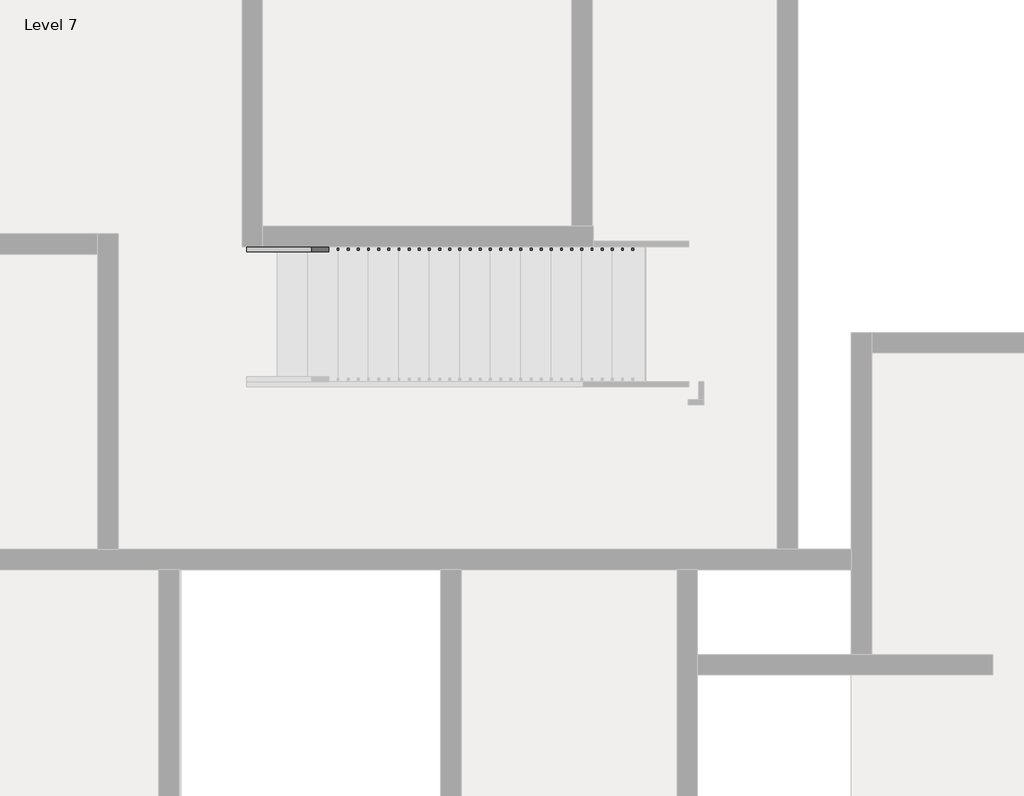
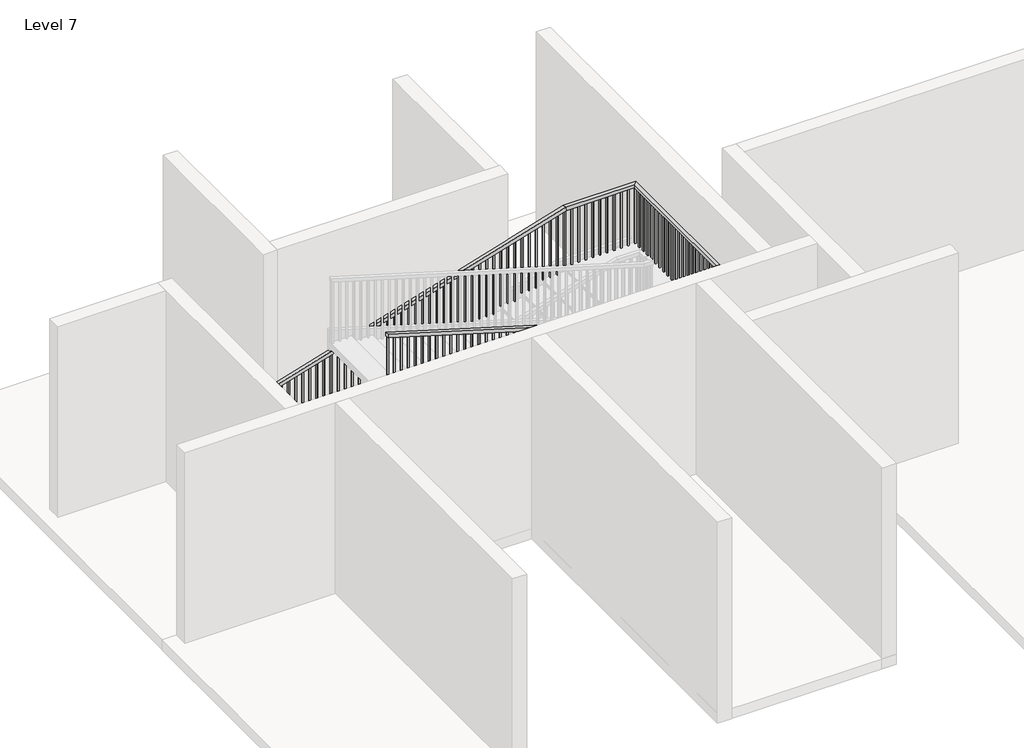
# One storey, part 10 of 14: 1 railing.
"""IFC4 building model written with IfcOpenShell, lengths in millimetres."""

from ifc_helpers import new_model, si_unit, frame, origin, place, context, project, spatial, polyline, outline, extrude, faceted_brep, element, save

model = new_model("IFC4")

# Units and contexts
model_context = context("Model", 3, world=origin())
ifc_project = project(units=[si_unit("LENGTHUNIT", "METRE", prefix="MILLI")], contexts=[model_context])

# Site, building, storey
site = spatial("IfcSite", under=ifc_project)
building = spatial("IfcBuilding", under=site)
storey = spatial("IfcBuildingStorey", under=building, Name="Level 7", Elevation=18288.0)

# Railing
placement = place(None, origin())
element("IfcRailing", 1, ObjectType="Handrail - Rectangular", at=placement, inside=storey, context=model_context, shape_type="SolidModel", body=[
    faceted_brep([(-5254.0891351, 12506.0715905, 19293.84), (-5254.0891351, 12506.0715905, 19240.8032429), (-5254.0891351, 12455.2715905, 19240.8032429), (-5254.0891351, 12455.2715905, 19293.84), (-986.8891351, 12506.0715905, 20574.0), (-979.4332782, 12506.0715905, 20523.2), (-979.4332782, 12455.2715905, 20523.2), (-986.8891351, 12455.2715905, 20574.0), (54.5108649, 12506.0715905, 20574.0), (54.5108649, 12506.0715905, 20523.2), (3.7108649, 12455.2715905, 20523.2), (3.7108649, 12455.2715905, 20574.0), (54.5108649, 9478.4949943, 20574.0), (54.5108649, 9478.4949943, 20523.2), (3.7108649, 9529.2949943, 20523.2), (3.7108649, 9529.2949943, 20574.0), (-682.0891351, 9478.4949943, 20574.0), (-689.544992, 9478.4949943, 20523.2), (-689.544992, 9529.2949943, 20523.2), (-682.0891351, 9529.2949943, 20574.0), (-5254.0891351, 9478.4949943, 21945.6), (-5254.0891351, 9529.2949943, 21945.6), (-5254.0891351, 9529.2949943, 21892.5632429), (-5254.0891351, 9478.4949943, 21892.5632429)], [[[0, 1, 2, 3]], [[1, 0, 4, 5]], [[2, 1, 5, 6]], [[3, 2, 6, 7]], [[0, 3, 7, 4]], [[5, 4, 8, 9]], [[6, 5, 9, 10]], [[7, 6, 10, 11]], [[4, 7, 11, 8]], [[9, 8, 12, 13]], [[10, 9, 13, 14]], [[11, 10, 14, 15]], [[8, 11, 15, 12]], [[13, 12, 16, 17]], [[14, 13, 17, 18]], [[15, 14, 18, 19]], [[12, 15, 19, 16]], [[20, 21, 22, 23]], [[17, 16, 20, 23]], [[18, 17, 23, 22]], [[19, 18, 22, 21]], [[16, 19, 21, 20]]]),
    extrude(outline(polyline([(21864.9407429, -5162.0141351), (20939.76, -5162.0141351), (20939.76, -5142.9641351), (21859.2257429, -5142.9641351), (21864.9407429, -5162.0141351)])), frame((0.0, 9494.3699943, 0.0), z_axis=(0.0, 1.0, 0.0), x_axis=(0.0, 0.0, 1.0)), (0.0, 0.0, 1.0), 19.05),
    extrude(outline(polyline([(21834.4607429, -5060.4141351), (20939.76, -5060.4141351), (20939.76, -5041.3641351), (21828.7457429, -5041.3641351), (21834.4607429, -5060.4141351)])), frame((0.0, 9494.3699943, 0.0), z_axis=(0.0, 1.0, 0.0), x_axis=(0.0, 0.0, 1.0)), (0.0, 0.0, 1.0), 19.05),
    extrude(outline(polyline([(21803.9807429, -4958.8141351), (20939.76, -4958.8141351), (20939.76, -4939.7641351), (21798.2657429, -4939.7641351), (21803.9807429, -4958.8141351)])), frame((0.0, 9494.3699943, 0.0), z_axis=(0.0, 1.0, 0.0), x_axis=(0.0, 0.0, 1.0)), (0.0, 0.0, 1.0), 19.05),
    extrude(outline(polyline([(21773.5007429, -4857.2141351), (20848.32, -4857.2141351), (20848.32, -4838.1641351), (21767.7857429, -4838.1641351), (21773.5007429, -4857.2141351)])), frame((0.0, 9494.3699943, 0.0), z_axis=(0.0, 1.0, 0.0), x_axis=(0.0, 0.0, 1.0)), (0.0, 0.0, 1.0), 19.05),
    extrude(outline(polyline([(21743.0207429, -4755.6141351), (20848.32, -4755.6141351), (20848.32, -4736.5641351), (21737.3057429, -4736.5641351), (21743.0207429, -4755.6141351)])), frame((0.0, 9494.3699943, 0.0), z_axis=(0.0, 1.0, 0.0), x_axis=(0.0, 0.0, 1.0)), (0.0, 0.0, 1.0), 19.05),
    extrude(outline(polyline([(21712.5407429, -4654.0141351), (20848.32, -4654.0141351), (20848.32, -4634.9641351), (21706.8257429, -4634.9641351), (21712.5407429, -4654.0141351)])), frame((0.0, 9494.3699943, 0.0), z_axis=(0.0, 1.0, 0.0), x_axis=(0.0, 0.0, 1.0)), (0.0, 0.0, 1.0), 19.05),
    extrude(outline(polyline([(21682.0607429, -4552.4141351), (20756.88, -4552.4141351), (20756.88, -4533.3641351), (21676.3457429, -4533.3641351), (21682.0607429, -4552.4141351)])), frame((0.0, 9494.3699943, 0.0), z_axis=(0.0, 1.0, 0.0), x_axis=(0.0, 0.0, 1.0)), (0.0, 0.0, 1.0), 19.05),
    extrude(outline(polyline([(21651.5807429, -4450.8141351), (20756.88, -4450.8141351), (20756.88, -4431.7641351), (21645.8657429, -4431.7641351), (21651.5807429, -4450.8141351)])), frame((0.0, 9494.3699943, 0.0), z_axis=(0.0, 1.0, 0.0), x_axis=(0.0, 0.0, 1.0)), (0.0, 0.0, 1.0), 19.05),
    extrude(outline(polyline([(21621.1007429, -4349.2141351), (20756.88, -4349.2141351), (20756.88, -4330.1641351), (21615.3857429, -4330.1641351), (21621.1007429, -4349.2141351)])), frame((0.0, 9494.3699943, 0.0), z_axis=(0.0, 1.0, 0.0), x_axis=(0.0, 0.0, 1.0)), (0.0, 0.0, 1.0), 19.05),
    extrude(outline(polyline([(21590.6207429, -4247.6141351), (20665.44, -4247.6141351), (20665.44, -4228.5641351), (21584.9057429, -4228.5641351), (21590.6207429, -4247.6141351)])), frame((0.0, 9494.3699943, 0.0), z_axis=(0.0, 1.0, 0.0), x_axis=(0.0, 0.0, 1.0)), (0.0, 0.0, 1.0), 19.05),
    extrude(outline(polyline([(21560.1407429, -4146.0141351), (20665.44, -4146.0141351), (20665.44, -4126.9641351), (21554.4257429, -4126.9641351), (21560.1407429, -4146.0141351)])), frame((0.0, 9494.3699943, 0.0), z_axis=(0.0, 1.0, 0.0), x_axis=(0.0, 0.0, 1.0)), (0.0, 0.0, 1.0), 19.05),
    extrude(outline(polyline([(21529.6607429, -4044.4141351), (20665.44, -4044.4141351), (20665.44, -4025.3641351), (21523.9457429, -4025.3641351), (21529.6607429, -4044.4141351)])), frame((0.0, 9494.3699943, 0.0), z_axis=(0.0, 1.0, 0.0), x_axis=(0.0, 0.0, 1.0)), (0.0, 0.0, 1.0), 19.05),
    extrude(outline(polyline([(21499.1807429, -3942.8141351), (20574.0, -3942.8141351), (20574.0, -3923.7641351), (21493.4657429, -3923.7641351), (21499.1807429, -3942.8141351)])), frame((0.0, 9494.3699943, 0.0), z_axis=(0.0, 1.0, 0.0), x_axis=(0.0, 0.0, 1.0)), (0.0, 0.0, 1.0), 19.05),
    extrude(outline(polyline([(21468.7007429, -3841.2141351), (20574.0, -3841.2141351), (20574.0, -3822.1641351), (21462.9857429, -3822.1641351), (21468.7007429, -3841.2141351)])), frame((0.0, 9494.3699943, 0.0), z_axis=(0.0, 1.0, 0.0), x_axis=(0.0, 0.0, 1.0)), (0.0, 0.0, 1.0), 19.05),
    extrude(outline(polyline([(21438.2207429, -3739.6141351), (20574.0, -3739.6141351), (20574.0, -3720.5641351), (21432.5057429, -3720.5641351), (21438.2207429, -3739.6141351)])), frame((0.0, 9494.3699943, 0.0), z_axis=(0.0, 1.0, 0.0), x_axis=(0.0, 0.0, 1.0)), (0.0, 0.0, 1.0), 19.05),
    extrude(outline(polyline([(21407.7407429, -3638.0141351), (20482.56, -3638.0141351), (20482.56, -3618.9641351), (21402.0257429, -3618.9641351), (21407.7407429, -3638.0141351)])), frame((0.0, 9494.3699943, 0.0), z_axis=(0.0, 1.0, 0.0), x_axis=(0.0, 0.0, 1.0)), (0.0, 0.0, 1.0), 19.05),
    extrude(outline(polyline([(21377.2607429, -3536.4141351), (20482.56, -3536.4141351), (20482.56, -3517.3641351), (21371.5457429, -3517.3641351), (21377.2607429, -3536.4141351)])), frame((0.0, 9494.3699943, 0.0), z_axis=(0.0, 1.0, 0.0), x_axis=(0.0, 0.0, 1.0)), (0.0, 0.0, 1.0), 19.05),
    extrude(outline(polyline([(21346.7807429, -3434.8141351), (20482.56, -3434.8141351), (20482.56, -3415.7641351), (21341.0657429, -3415.7641351), (21346.7807429, -3434.8141351)])), frame((0.0, 9494.3699943, 0.0), z_axis=(0.0, 1.0, 0.0), x_axis=(0.0, 0.0, 1.0)), (0.0, 0.0, 1.0), 19.05),
    extrude(outline(polyline([(21316.3007429, -3333.2141351), (20391.12, -3333.2141351), (20391.12, -3314.1641351), (21310.5857429, -3314.1641351), (21316.3007429, -3333.2141351)])), frame((0.0, 9494.3699943, 0.0), z_axis=(0.0, 1.0, 0.0), x_axis=(0.0, 0.0, 1.0)), (0.0, 0.0, 1.0), 19.05),
    extrude(outline(polyline([(21285.8207429, -3231.6141351), (20391.12, -3231.6141351), (20391.12, -3212.5641351), (21280.1057429, -3212.5641351), (21285.8207429, -3231.6141351)])), frame((0.0, 9494.3699943, 0.0), z_axis=(0.0, 1.0, 0.0), x_axis=(0.0, 0.0, 1.0)), (0.0, 0.0, 1.0), 19.05),
    extrude(outline(polyline([(21255.3407429, -3130.0141351), (20391.12, -3130.0141351), (20391.12, -3110.9641351), (21249.6257429, -3110.9641351), (21255.3407429, -3130.0141351)])), frame((0.0, 9494.3699943, 0.0), z_axis=(0.0, 1.0, 0.0), x_axis=(0.0, 0.0, 1.0)), (0.0, 0.0, 1.0), 19.05),
    extrude(outline(polyline([(21224.8607429, -3028.4141351), (20299.68, -3028.4141351), (20299.68, -3009.3641351), (21219.1457429, -3009.3641351), (21224.8607429, -3028.4141351)])), frame((0.0, 9494.3699943, 0.0), z_axis=(0.0, 1.0, 0.0), x_axis=(0.0, 0.0, 1.0)), (0.0, 0.0, 1.0), 19.05),
    extrude(outline(polyline([(21194.3807429, -2926.8141351), (20299.68, -2926.8141351), (20299.68, -2907.7641351), (21188.6657429, -2907.7641351), (21194.3807429, -2926.8141351)])), frame((0.0, 9494.3699943, 0.0), z_axis=(0.0, 1.0, 0.0), x_axis=(0.0, 0.0, 1.0)), (0.0, 0.0, 1.0), 19.05),
    extrude(outline(polyline([(21163.9007429, -2825.2141351), (20299.68, -2825.2141351), (20299.68, -2806.1641351), (21158.1857429, -2806.1641351), (21163.9007429, -2825.2141351)])), frame((0.0, 9494.3699943, 0.0), z_axis=(0.0, 1.0, 0.0), x_axis=(0.0, 0.0, 1.0)), (0.0, 0.0, 1.0), 19.05),
    extrude(outline(polyline([(21133.4207429, -2723.6141351), (20208.24, -2723.6141351), (20208.24, -2704.5641351), (21127.7057429, -2704.5641351), (21133.4207429, -2723.6141351)])), frame((0.0, 9494.3699943, 0.0), z_axis=(0.0, 1.0, 0.0), x_axis=(0.0, 0.0, 1.0)), (0.0, 0.0, 1.0), 19.05),
    extrude(outline(polyline([(21102.9407429, -2622.0141351), (20208.24, -2622.0141351), (20208.24, -2602.9641351), (21097.2257429, -2602.9641351), (21102.9407429, -2622.0141351)])), frame((0.0, 9494.3699943, 0.0), z_axis=(0.0, 1.0, 0.0), x_axis=(0.0, 0.0, 1.0)), (0.0, 0.0, 1.0), 19.05),
    extrude(outline(polyline([(21072.4607429, -2520.4141351), (20208.24, -2520.4141351), (20208.24, -2501.3641351), (21066.7457429, -2501.3641351), (21072.4607429, -2520.4141351)])), frame((0.0, 9494.3699943, 0.0), z_axis=(0.0, 1.0, 0.0), x_axis=(0.0, 0.0, 1.0)), (0.0, 0.0, 1.0), 19.05),
    extrude(outline(polyline([(21041.9807429, -2418.8141351), (20116.8, -2418.8141351), (20116.8, -2399.7641351), (21036.2657429, -2399.7641351), (21041.9807429, -2418.8141351)])), frame((0.0, 9494.3699943, 0.0), z_axis=(0.0, 1.0, 0.0), x_axis=(0.0, 0.0, 1.0)), (0.0, 0.0, 1.0), 19.05),
    extrude(outline(polyline([(21011.5007429, -2317.2141351), (20116.8, -2317.2141351), (20116.8, -2298.1641351), (21005.7857429, -2298.1641351), (21011.5007429, -2317.2141351)])), frame((0.0, 9494.3699943, 0.0), z_axis=(0.0, 1.0, 0.0), x_axis=(0.0, 0.0, 1.0)), (0.0, 0.0, 1.0), 19.05),
    extrude(outline(polyline([(20981.0207429, -2215.6141351), (20116.8, -2215.6141351), (20116.8, -2196.5641351), (20975.3057429, -2196.5641351), (20981.0207429, -2215.6141351)])), frame((0.0, 9494.3699943, 0.0), z_axis=(0.0, 1.0, 0.0), x_axis=(0.0, 0.0, 1.0)), (0.0, 0.0, 1.0), 19.05),
    extrude(outline(polyline([(20950.5407429, -2114.0141351), (20025.36, -2114.0141351), (20025.36, -2094.9641351), (20944.8257429, -2094.9641351), (20950.5407429, -2114.0141351)])), frame((0.0, 9494.3699943, 0.0), z_axis=(0.0, 1.0, 0.0), x_axis=(0.0, 0.0, 1.0)), (0.0, 0.0, 1.0), 19.05),
    extrude(outline(polyline([(20920.0607429, -2012.4141351), (20025.36, -2012.4141351), (20025.36, -1993.3641351), (20914.3457429, -1993.3641351), (20920.0607429, -2012.4141351)])), frame((0.0, 9494.3699943, 0.0), z_axis=(0.0, 1.0, 0.0), x_axis=(0.0, 0.0, 1.0)), (0.0, 0.0, 1.0), 19.05),
    extrude(outline(polyline([(20889.5807429, -1910.8141351), (20025.36, -1910.8141351), (20025.36, -1891.7641351), (20883.8657429, -1891.7641351), (20889.5807429, -1910.8141351)])), frame((0.0, 9494.3699943, 0.0), z_axis=(0.0, 1.0, 0.0), x_axis=(0.0, 0.0, 1.0)), (0.0, 0.0, 1.0), 19.05),
    extrude(outline(polyline([(20859.1007429, -1809.2141351), (19933.92, -1809.2141351), (19933.92, -1790.1641351), (20853.3857429, -1790.1641351), (20859.1007429, -1809.2141351)])), frame((0.0, 9494.3699943, 0.0), z_axis=(0.0, 1.0, 0.0), x_axis=(0.0, 0.0, 1.0)), (0.0, 0.0, 1.0), 19.05),
    extrude(outline(polyline([(20828.6207429, -1707.6141351), (19933.92, -1707.6141351), (19933.92, -1688.5641351), (20822.9057429, -1688.5641351), (20828.6207429, -1707.6141351)])), frame((0.0, 9494.3699943, 0.0), z_axis=(0.0, 1.0, 0.0), x_axis=(0.0, 0.0, 1.0)), (0.0, 0.0, 1.0), 19.05),
    extrude(outline(polyline([(20798.1407429, -1606.0141351), (19933.92, -1606.0141351), (19933.92, -1586.9641351), (20792.4257429, -1586.9641351), (20798.1407429, -1606.0141351)])), frame((0.0, 9494.3699943, 0.0), z_axis=(0.0, 1.0, 0.0), x_axis=(0.0, 0.0, 1.0)), (0.0, 0.0, 1.0), 19.05),
    extrude(outline(polyline([(20767.6607429, -1504.4141351), (19842.48, -1504.4141351), (19842.48, -1485.3641351), (20761.9457429, -1485.3641351), (20767.6607429, -1504.4141351)])), frame((0.0, 9494.3699943, 0.0), z_axis=(0.0, 1.0, 0.0), x_axis=(0.0, 0.0, 1.0)), (0.0, 0.0, 1.0), 19.05),
    extrude(outline(polyline([(20737.1807429, -1402.8141351), (19842.48, -1402.8141351), (19842.48, -1383.7641351), (20731.4657429, -1383.7641351), (20737.1807429, -1402.8141351)])), frame((0.0, 9494.3699943, 0.0), z_axis=(0.0, 1.0, 0.0), x_axis=(0.0, 0.0, 1.0)), (0.0, 0.0, 1.0), 19.05),
    extrude(outline(polyline([(20706.7007429, -1301.2141351), (19842.48, -1301.2141351), (19842.48, -1282.1641351), (20700.9857429, -1282.1641351), (20706.7007429, -1301.2141351)])), frame((0.0, 9494.3699943, 0.0), z_axis=(0.0, 1.0, 0.0), x_axis=(0.0, 0.0, 1.0)), (0.0, 0.0, 1.0), 19.05),
    extrude(outline(polyline([(20676.2207429, -1199.6141351), (19751.04, -1199.6141351), (19751.04, -1180.5641351), (20670.5057429, -1180.5641351), (20676.2207429, -1199.6141351)])), frame((0.0, 9494.3699943, 0.0), z_axis=(0.0, 1.0, 0.0), x_axis=(0.0, 0.0, 1.0)), (0.0, 0.0, 1.0), 19.05),
    extrude(outline(polyline([(20645.7407429, -1098.0141351), (19751.04, -1098.0141351), (19751.04, -1078.9641351), (20640.0257429, -1078.9641351), (20645.7407429, -1098.0141351)])), frame((0.0, 9494.3699943, 0.0), z_axis=(0.0, 1.0, 0.0), x_axis=(0.0, 0.0, 1.0)), (0.0, 0.0, 1.0), 19.05),
    extrude(outline(polyline([(20615.2607429, -996.4141351), (19751.04, -996.4141351), (19751.04, -977.3641351), (20609.5457429, -977.3641351), (20615.2607429, -996.4141351)])), frame((0.0, 9494.3699943, 0.0), z_axis=(0.0, 1.0, 0.0), x_axis=(0.0, 0.0, 1.0)), (0.0, 0.0, 1.0), 19.05),
    extrude(outline(polyline([(20584.7807429, -894.8141351), (19659.6, -894.8141351), (19659.6, -875.7641351), (20579.0657429, -875.7641351), (20584.7807429, -894.8141351)])), frame((0.0, 9494.3699943, 0.0), z_axis=(0.0, 1.0, 0.0), x_axis=(0.0, 0.0, 1.0)), (0.0, 0.0, 1.0), 19.05),
    extrude(outline(polyline([(20554.3007429, -793.2141351), (19659.6, -793.2141351), (19659.6, -774.1641351), (20548.5857429, -774.1641351), (20554.3007429, -793.2141351)])), frame((0.0, 9494.3699943, 0.0), z_axis=(0.0, 1.0, 0.0), x_axis=(0.0, 0.0, 1.0)), (0.0, 0.0, 1.0), 19.05),
    extrude(outline(polyline([(-672.5641351, 9494.3699943), (-691.6141351, 9494.3699943), (-691.6141351, 9513.4199943), (-672.5641351, 9513.4199943), (-672.5641351, 9494.3699943)])), frame((0.0, 0.0, 19659.6), z_axis=(0.0, 0.0, 1.0), x_axis=(1.0, 0.0, 0.0)), (0.0, 0.0, 1.0), 863.6),
    extrude(outline(polyline([(-570.9641351, 9494.3699943), (-590.0141351, 9494.3699943), (-590.0141351, 9513.4199943), (-570.9641351, 9513.4199943), (-570.9641351, 9494.3699943)])), frame((0.0, 0.0, 19659.6), z_axis=(0.0, 0.0, 1.0), x_axis=(1.0, 0.0, 0.0)), (0.0, 0.0, 1.0), 863.6),
    extrude(outline(polyline([(-469.3641351, 9494.3699943), (-488.4141351, 9494.3699943), (-488.4141351, 9513.4199943), (-469.3641351, 9513.4199943), (-469.3641351, 9494.3699943)])), frame((0.0, 0.0, 19659.6), z_axis=(0.0, 0.0, 1.0), x_axis=(1.0, 0.0, 0.0)), (0.0, 0.0, 1.0), 863.6),
    extrude(outline(polyline([(-367.7641351, 9494.3699943), (-386.8141351, 9494.3699943), (-386.8141351, 9513.4199943), (-367.7641351, 9513.4199943), (-367.7641351, 9494.3699943)])), frame((0.0, 0.0, 19659.6), z_axis=(0.0, 0.0, 1.0), x_axis=(1.0, 0.0, 0.0)), (0.0, 0.0, 1.0), 863.6),
    extrude(outline(polyline([(-266.1641351, 9494.3699943), (-285.2141351, 9494.3699943), (-285.2141351, 9513.4199943), (-266.1641351, 9513.4199943), (-266.1641351, 9494.3699943)])), frame((0.0, 0.0, 19659.6), z_axis=(0.0, 0.0, 1.0), x_axis=(1.0, 0.0, 0.0)), (0.0, 0.0, 1.0), 863.6),
    extrude(outline(polyline([(-164.5641351, 9494.3699943), (-183.6141351, 9494.3699943), (-183.6141351, 9513.4199943), (-164.5641351, 9513.4199943), (-164.5641351, 9494.3699943)])), frame((0.0, 0.0, 19659.6), z_axis=(0.0, 0.0, 1.0), x_axis=(1.0, 0.0, 0.0)), (0.0, 0.0, 1.0), 863.6),
    extrude(outline(polyline([(-62.9641351, 9494.3699943), (-82.0141351, 9494.3699943), (-82.0141351, 9513.4199943), (-62.9641351, 9513.4199943), (-62.9641351, 9494.3699943)])), frame((0.0, 0.0, 19659.6), z_axis=(0.0, 0.0, 1.0), x_axis=(1.0, 0.0, 0.0)), (0.0, 0.0, 1.0), 863.6),
    extrude(outline(polyline([(38.6358649, 9543.7965905), (38.6358649, 9524.7465905), (19.5858649, 9524.7465905), (19.5858649, 9543.7965905), (38.6358649, 9543.7965905)])), frame((0.0, 0.0, 19659.6), z_axis=(0.0, 0.0, 1.0), x_axis=(1.0, 0.0, 0.0)), (0.0, 0.0, 1.0), 863.6),
    extrude(outline(polyline([(38.6358649, 9645.3965905), (38.6358649, 9626.3465905), (19.5858649, 9626.3465905), (19.5858649, 9645.3965905), (38.6358649, 9645.3965905)])), frame((0.0, 0.0, 19659.6), z_axis=(0.0, 0.0, 1.0), x_axis=(1.0, 0.0, 0.0)), (0.0, 0.0, 1.0), 863.6),
    extrude(outline(polyline([(38.6358649, 9746.9965905), (38.6358649, 9727.9465905), (19.5858649, 9727.9465905), (19.5858649, 9746.9965905), (38.6358649, 9746.9965905)])), frame((0.0, 0.0, 19659.6), z_axis=(0.0, 0.0, 1.0), x_axis=(1.0, 0.0, 0.0)), (0.0, 0.0, 1.0), 863.6),
    extrude(outline(polyline([(38.6358649, 9848.5965905), (38.6358649, 9829.5465905), (19.5858649, 9829.5465905), (19.5858649, 9848.5965905), (38.6358649, 9848.5965905)])), frame((0.0, 0.0, 19659.6), z_axis=(0.0, 0.0, 1.0), x_axis=(1.0, 0.0, 0.0)), (0.0, 0.0, 1.0), 863.6),
    extrude(outline(polyline([(38.6358649, 9950.1965905), (38.6358649, 9931.1465905), (19.5858649, 9931.1465905), (19.5858649, 9950.1965905), (38.6358649, 9950.1965905)])), frame((0.0, 0.0, 19659.6), z_axis=(0.0, 0.0, 1.0), x_axis=(1.0, 0.0, 0.0)), (0.0, 0.0, 1.0), 863.6),
    extrude(outline(polyline([(38.6358649, 10051.7965905), (38.6358649, 10032.7465905), (19.5858649, 10032.7465905), (19.5858649, 10051.7965905), (38.6358649, 10051.7965905)])), frame((0.0, 0.0, 19659.6), z_axis=(0.0, 0.0, 1.0), x_axis=(1.0, 0.0, 0.0)), (0.0, 0.0, 1.0), 863.6),
    extrude(outline(polyline([(38.6358649, 10153.3965905), (38.6358649, 10134.3465905), (19.5858649, 10134.3465905), (19.5858649, 10153.3965905), (38.6358649, 10153.3965905)])), frame((0.0, 0.0, 19659.6), z_axis=(0.0, 0.0, 1.0), x_axis=(1.0, 0.0, 0.0)), (0.0, 0.0, 1.0), 863.6),
    extrude(outline(polyline([(38.6358649, 10254.9965905), (38.6358649, 10235.9465905), (19.5858649, 10235.9465905), (19.5858649, 10254.9965905), (38.6358649, 10254.9965905)])), frame((0.0, 0.0, 19659.6), z_axis=(0.0, 0.0, 1.0), x_axis=(1.0, 0.0, 0.0)), (0.0, 0.0, 1.0), 863.6),
    extrude(outline(polyline([(38.6358649, 10356.5965905), (38.6358649, 10337.5465905), (19.5858649, 10337.5465905), (19.5858649, 10356.5965905), (38.6358649, 10356.5965905)])), frame((0.0, 0.0, 19659.6), z_axis=(0.0, 0.0, 1.0), x_axis=(1.0, 0.0, 0.0)), (0.0, 0.0, 1.0), 863.6),
    extrude(outline(polyline([(38.6358649, 10458.1965905), (38.6358649, 10439.1465905), (19.5858649, 10439.1465905), (19.5858649, 10458.1965905), (38.6358649, 10458.1965905)])), frame((0.0, 0.0, 19659.6), z_axis=(0.0, 0.0, 1.0), x_axis=(1.0, 0.0, 0.0)), (0.0, 0.0, 1.0), 863.6),
    extrude(outline(polyline([(38.6358649, 10559.7965905), (38.6358649, 10540.7465905), (19.5858649, 10540.7465905), (19.5858649, 10559.7965905), (38.6358649, 10559.7965905)])), frame((0.0, 0.0, 19659.6), z_axis=(0.0, 0.0, 1.0), x_axis=(1.0, 0.0, 0.0)), (0.0, 0.0, 1.0), 863.6),
    extrude(outline(polyline([(38.6358649, 10661.3965905), (38.6358649, 10642.3465905), (19.5858649, 10642.3465905), (19.5858649, 10661.3965905), (38.6358649, 10661.3965905)])), frame((0.0, 0.0, 19659.6), z_axis=(0.0, 0.0, 1.0), x_axis=(1.0, 0.0, 0.0)), (0.0, 0.0, 1.0), 863.6),
    extrude(outline(polyline([(38.6358649, 10762.9965905), (38.6358649, 10743.9465905), (19.5858649, 10743.9465905), (19.5858649, 10762.9965905), (38.6358649, 10762.9965905)])), frame((0.0, 0.0, 19659.6), z_axis=(0.0, 0.0, 1.0), x_axis=(1.0, 0.0, 0.0)), (0.0, 0.0, 1.0), 863.6),
    extrude(outline(polyline([(38.6358649, 10864.5965905), (38.6358649, 10845.5465905), (19.5858649, 10845.5465905), (19.5858649, 10864.5965905), (38.6358649, 10864.5965905)])), frame((0.0, 0.0, 19659.6), z_axis=(0.0, 0.0, 1.0), x_axis=(1.0, 0.0, 0.0)), (0.0, 0.0, 1.0), 863.6),
    extrude(outline(polyline([(38.6358649, 10966.1965905), (38.6358649, 10947.1465905), (19.5858649, 10947.1465905), (19.5858649, 10966.1965905), (38.6358649, 10966.1965905)])), frame((0.0, 0.0, 19659.6), z_axis=(0.0, 0.0, 1.0), x_axis=(1.0, 0.0, 0.0)), (0.0, 0.0, 1.0), 863.6),
    extrude(outline(polyline([(38.6358649, 11067.7965905), (38.6358649, 11048.7465905), (19.5858649, 11048.7465905), (19.5858649, 11067.7965905), (38.6358649, 11067.7965905)])), frame((0.0, 0.0, 19659.6), z_axis=(0.0, 0.0, 1.0), x_axis=(1.0, 0.0, 0.0)), (0.0, 0.0, 1.0), 863.6),
    extrude(outline(polyline([(38.6358649, 11169.3965905), (38.6358649, 11150.3465905), (19.5858649, 11150.3465905), (19.5858649, 11169.3965905), (38.6358649, 11169.3965905)])), frame((0.0, 0.0, 19659.6), z_axis=(0.0, 0.0, 1.0), x_axis=(1.0, 0.0, 0.0)), (0.0, 0.0, 1.0), 863.6),
    extrude(outline(polyline([(38.6358649, 11270.9965905), (38.6358649, 11251.9465905), (19.5858649, 11251.9465905), (19.5858649, 11270.9965905), (38.6358649, 11270.9965905)])), frame((0.0, 0.0, 19659.6), z_axis=(0.0, 0.0, 1.0), x_axis=(1.0, 0.0, 0.0)), (0.0, 0.0, 1.0), 863.6),
    extrude(outline(polyline([(38.6358649, 11372.5965905), (38.6358649, 11353.5465905), (19.5858649, 11353.5465905), (19.5858649, 11372.5965905), (38.6358649, 11372.5965905)])), frame((0.0, 0.0, 19659.6), z_axis=(0.0, 0.0, 1.0), x_axis=(1.0, 0.0, 0.0)), (0.0, 0.0, 1.0), 863.6),
    extrude(outline(polyline([(38.6358649, 11474.1965905), (38.6358649, 11455.1465905), (19.5858649, 11455.1465905), (19.5858649, 11474.1965905), (38.6358649, 11474.1965905)])), frame((0.0, 0.0, 19659.6), z_axis=(0.0, 0.0, 1.0), x_axis=(1.0, 0.0, 0.0)), (0.0, 0.0, 1.0), 863.6),
    extrude(outline(polyline([(38.6358649, 11575.7965905), (38.6358649, 11556.7465905), (19.5858649, 11556.7465905), (19.5858649, 11575.7965905), (38.6358649, 11575.7965905)])), frame((0.0, 0.0, 19659.6), z_axis=(0.0, 0.0, 1.0), x_axis=(1.0, 0.0, 0.0)), (0.0, 0.0, 1.0), 863.6),
    extrude(outline(polyline([(38.6358649, 11677.3965905), (38.6358649, 11658.3465905), (19.5858649, 11658.3465905), (19.5858649, 11677.3965905), (38.6358649, 11677.3965905)])), frame((0.0, 0.0, 19659.6), z_axis=(0.0, 0.0, 1.0), x_axis=(1.0, 0.0, 0.0)), (0.0, 0.0, 1.0), 863.6),
    extrude(outline(polyline([(38.6358649, 11778.9965905), (38.6358649, 11759.9465905), (19.5858649, 11759.9465905), (19.5858649, 11778.9965905), (38.6358649, 11778.9965905)])), frame((0.0, 0.0, 19659.6), z_axis=(0.0, 0.0, 1.0), x_axis=(1.0, 0.0, 0.0)), (0.0, 0.0, 1.0), 863.6),
    extrude(outline(polyline([(38.6358649, 11880.5965905), (38.6358649, 11861.5465905), (19.5858649, 11861.5465905), (19.5858649, 11880.5965905), (38.6358649, 11880.5965905)])), frame((0.0, 0.0, 19659.6), z_axis=(0.0, 0.0, 1.0), x_axis=(1.0, 0.0, 0.0)), (0.0, 0.0, 1.0), 863.6),
    extrude(outline(polyline([(38.6358649, 11982.1965905), (38.6358649, 11963.1465905), (19.5858649, 11963.1465905), (19.5858649, 11982.1965905), (38.6358649, 11982.1965905)])), frame((0.0, 0.0, 19659.6), z_axis=(0.0, 0.0, 1.0), x_axis=(1.0, 0.0, 0.0)), (0.0, 0.0, 1.0), 863.6),
    extrude(outline(polyline([(38.6358649, 12083.7965905), (38.6358649, 12064.7465905), (19.5858649, 12064.7465905), (19.5858649, 12083.7965905), (38.6358649, 12083.7965905)])), frame((0.0, 0.0, 19659.6), z_axis=(0.0, 0.0, 1.0), x_axis=(1.0, 0.0, 0.0)), (0.0, 0.0, 1.0), 863.6),
    extrude(outline(polyline([(38.6358649, 12185.3965905), (38.6358649, 12166.3465905), (19.5858649, 12166.3465905), (19.5858649, 12185.3965905), (38.6358649, 12185.3965905)])), frame((0.0, 0.0, 19659.6), z_axis=(0.0, 0.0, 1.0), x_axis=(1.0, 0.0, 0.0)), (0.0, 0.0, 1.0), 863.6),
    extrude(outline(polyline([(38.6358649, 12286.9965905), (38.6358649, 12267.9465905), (19.5858649, 12267.9465905), (19.5858649, 12286.9965905), (38.6358649, 12286.9965905)])), frame((0.0, 0.0, 19659.6), z_axis=(0.0, 0.0, 1.0), x_axis=(1.0, 0.0, 0.0)), (0.0, 0.0, 1.0), 863.6),
    extrude(outline(polyline([(38.6358649, 12388.5965905), (38.6358649, 12369.5465905), (19.5858649, 12369.5465905), (19.5858649, 12388.5965905), (38.6358649, 12388.5965905)])), frame((0.0, 0.0, 19659.6), z_axis=(0.0, 0.0, 1.0), x_axis=(1.0, 0.0, 0.0)), (0.0, 0.0, 1.0), 863.6),
    extrude(outline(polyline([(-82.0141351, 12490.1965905), (-62.9641351, 12490.1965905), (-62.9641351, 12471.1465905), (-82.0141351, 12471.1465905), (-82.0141351, 12490.1965905)])), frame((0.0, 0.0, 19659.6), z_axis=(0.0, 0.0, 1.0), x_axis=(1.0, 0.0, 0.0)), (0.0, 0.0, 1.0), 863.6),
    extrude(outline(polyline([(-183.6141351, 12490.1965905), (-164.5641351, 12490.1965905), (-164.5641351, 12471.1465905), (-183.6141351, 12471.1465905), (-183.6141351, 12490.1965905)])), frame((0.0, 0.0, 19659.6), z_axis=(0.0, 0.0, 1.0), x_axis=(1.0, 0.0, 0.0)), (0.0, 0.0, 1.0), 863.6),
    extrude(outline(polyline([(-285.2141351, 12490.1965905), (-266.1641351, 12490.1965905), (-266.1641351, 12471.1465905), (-285.2141351, 12471.1465905), (-285.2141351, 12490.1965905)])), frame((0.0, 0.0, 19659.6), z_axis=(0.0, 0.0, 1.0), x_axis=(1.0, 0.0, 0.0)), (0.0, 0.0, 1.0), 863.6),
    extrude(outline(polyline([(-386.8141351, 12490.1965905), (-367.7641351, 12490.1965905), (-367.7641351, 12471.1465905), (-386.8141351, 12471.1465905), (-386.8141351, 12490.1965905)])), frame((0.0, 0.0, 19659.6), z_axis=(0.0, 0.0, 1.0), x_axis=(1.0, 0.0, 0.0)), (0.0, 0.0, 1.0), 863.6),
    extrude(outline(polyline([(-488.4141351, 12490.1965905), (-469.3641351, 12490.1965905), (-469.3641351, 12471.1465905), (-488.4141351, 12471.1465905), (-488.4141351, 12490.1965905)])), frame((0.0, 0.0, 19659.6), z_axis=(0.0, 0.0, 1.0), x_axis=(1.0, 0.0, 0.0)), (0.0, 0.0, 1.0), 863.6),
    extrude(outline(polyline([(-590.0141351, 12490.1965905), (-570.9641351, 12490.1965905), (-570.9641351, 12471.1465905), (-590.0141351, 12471.1465905), (-590.0141351, 12490.1965905)])), frame((0.0, 0.0, 19659.6), z_axis=(0.0, 0.0, 1.0), x_axis=(1.0, 0.0, 0.0)), (0.0, 0.0, 1.0), 863.6),
    extrude(outline(polyline([(-691.6141351, 12490.1965905), (-672.5641351, 12490.1965905), (-672.5641351, 12471.1465905), (-691.6141351, 12471.1465905), (-691.6141351, 12490.1965905)])), frame((0.0, 0.0, 19659.6), z_axis=(0.0, 0.0, 1.0), x_axis=(1.0, 0.0, 0.0)), (0.0, 0.0, 1.0), 863.6),
    extrude(outline(polyline([(-793.2141351, 12490.1965905), (-774.1641351, 12490.1965905), (-774.1641351, 12471.1465905), (-793.2141351, 12471.1465905), (-793.2141351, 12490.1965905)])), frame((0.0, 0.0, 19659.6), z_axis=(0.0, 0.0, 1.0), x_axis=(1.0, 0.0, 0.0)), (0.0, 0.0, 1.0), 863.6),
    extrude(outline(polyline([(-894.8141351, 12490.1965905), (-875.7641351, 12490.1965905), (-875.7641351, 12471.1465905), (-894.8141351, 12471.1465905), (-894.8141351, 12490.1965905)])), frame((0.0, 0.0, 19659.6), z_axis=(0.0, 0.0, 1.0), x_axis=(1.0, 0.0, 0.0)), (0.0, 0.0, 1.0), 863.6),
    extrude(outline(polyline([(20518.1057429, -996.4141351), (19659.6, -996.4141351), (19659.6, -977.3641351), (20523.8207429, -977.3641351), (20518.1057429, -996.4141351)])), frame((0.0, 12471.1465905, 0.0), z_axis=(0.0, 1.0, 0.0), x_axis=(0.0, 0.0, 1.0)), (0.0, 0.0, 1.0), 19.05),
    extrude(outline(polyline([(20487.6257429, -1098.0141351), (19568.16, -1098.0141351), (19568.16, -1078.9641351), (20493.3407429, -1078.9641351), (20487.6257429, -1098.0141351)])), frame((0.0, 12471.1465905, 0.0), z_axis=(0.0, 1.0, 0.0), x_axis=(0.0, 0.0, 1.0)), (0.0, 0.0, 1.0), 19.05),
    extrude(outline(polyline([(20457.1457429, -1199.6141351), (19568.16, -1199.6141351), (19568.16, -1180.5641351), (20462.8607429, -1180.5641351), (20457.1457429, -1199.6141351)])), frame((0.0, 12471.1465905, 0.0), z_axis=(0.0, 1.0, 0.0), x_axis=(0.0, 0.0, 1.0)), (0.0, 0.0, 1.0), 19.05),
    extrude(outline(polyline([(20426.6657429, -1301.2141351), (19568.16, -1301.2141351), (19568.16, -1282.1641351), (20432.3807429, -1282.1641351), (20426.6657429, -1301.2141351)])), frame((0.0, 12471.1465905, 0.0), z_axis=(0.0, 1.0, 0.0), x_axis=(0.0, 0.0, 1.0)), (0.0, 0.0, 1.0), 19.05),
    extrude(outline(polyline([(20396.1857429, -1402.8141351), (19476.72, -1402.8141351), (19476.72, -1383.7641351), (20401.9007429, -1383.7641351), (20396.1857429, -1402.8141351)])), frame((0.0, 12471.1465905, 0.0), z_axis=(0.0, 1.0, 0.0), x_axis=(0.0, 0.0, 1.0)), (0.0, 0.0, 1.0), 19.05),
    extrude(outline(polyline([(20365.7057429, -1504.4141351), (19476.72, -1504.4141351), (19476.72, -1485.3641351), (20371.4207429, -1485.3641351), (20365.7057429, -1504.4141351)])), frame((0.0, 12471.1465905, 0.0), z_axis=(0.0, 1.0, 0.0), x_axis=(0.0, 0.0, 1.0)), (0.0, 0.0, 1.0), 19.05),
    extrude(outline(polyline([(20335.2257429, -1606.0141351), (19476.72, -1606.0141351), (19476.72, -1586.9641351), (20340.9407429, -1586.9641351), (20335.2257429, -1606.0141351)])), frame((0.0, 12471.1465905, 0.0), z_axis=(0.0, 1.0, 0.0), x_axis=(0.0, 0.0, 1.0)), (0.0, 0.0, 1.0), 19.05),
    extrude(outline(polyline([(20304.7457429, -1707.6141351), (19385.28, -1707.6141351), (19385.28, -1688.5641351), (20310.4607429, -1688.5641351), (20304.7457429, -1707.6141351)])), frame((0.0, 12471.1465905, 0.0), z_axis=(0.0, 1.0, 0.0), x_axis=(0.0, 0.0, 1.0)), (0.0, 0.0, 1.0), 19.05),
    extrude(outline(polyline([(20274.2657429, -1809.2141351), (19385.28, -1809.2141351), (19385.28, -1790.1641351), (20279.9807429, -1790.1641351), (20274.2657429, -1809.2141351)])), frame((0.0, 12471.1465905, 0.0), z_axis=(0.0, 1.0, 0.0), x_axis=(0.0, 0.0, 1.0)), (0.0, 0.0, 1.0), 19.05),
    extrude(outline(polyline([(20243.7857429, -1910.8141351), (19385.28, -1910.8141351), (19385.28, -1891.7641351), (20249.5007429, -1891.7641351), (20243.7857429, -1910.8141351)])), frame((0.0, 12471.1465905, 0.0), z_axis=(0.0, 1.0, 0.0), x_axis=(0.0, 0.0, 1.0)), (0.0, 0.0, 1.0), 19.05),
    extrude(outline(polyline([(20213.3057429, -2012.4141351), (19293.84, -2012.4141351), (19293.84, -1993.3641351), (20219.0207429, -1993.3641351), (20213.3057429, -2012.4141351)])), frame((0.0, 12471.1465905, 0.0), z_axis=(0.0, 1.0, 0.0), x_axis=(0.0, 0.0, 1.0)), (0.0, 0.0, 1.0), 19.05),
    extrude(outline(polyline([(20182.8257429, -2114.0141351), (19293.84, -2114.0141351), (19293.84, -2094.9641351), (20188.5407429, -2094.9641351), (20182.8257429, -2114.0141351)])), frame((0.0, 12471.1465905, 0.0), z_axis=(0.0, 1.0, 0.0), x_axis=(0.0, 0.0, 1.0)), (0.0, 0.0, 1.0), 19.05),
    extrude(outline(polyline([(20152.3457429, -2215.6141351), (19293.84, -2215.6141351), (19293.84, -2196.5641351), (20158.0607429, -2196.5641351), (20152.3457429, -2215.6141351)])), frame((0.0, 12471.1465905, 0.0), z_axis=(0.0, 1.0, 0.0), x_axis=(0.0, 0.0, 1.0)), (0.0, 0.0, 1.0), 19.05),
    extrude(outline(polyline([(20121.8657429, -2317.2141351), (19202.4, -2317.2141351), (19202.4, -2298.1641351), (20127.5807429, -2298.1641351), (20121.8657429, -2317.2141351)])), frame((0.0, 12471.1465905, 0.0), z_axis=(0.0, 1.0, 0.0), x_axis=(0.0, 0.0, 1.0)), (0.0, 0.0, 1.0), 19.05),
    extrude(outline(polyline([(20091.3857429, -2418.8141351), (19202.4, -2418.8141351), (19202.4, -2399.7641351), (20097.1007429, -2399.7641351), (20091.3857429, -2418.8141351)])), frame((0.0, 12471.1465905, 0.0), z_axis=(0.0, 1.0, 0.0), x_axis=(0.0, 0.0, 1.0)), (0.0, 0.0, 1.0), 19.05),
    extrude(outline(polyline([(20060.9057429, -2520.4141351), (19202.4, -2520.4141351), (19202.4, -2501.3641351), (20066.6207429, -2501.3641351), (20060.9057429, -2520.4141351)])), frame((0.0, 12471.1465905, 0.0), z_axis=(0.0, 1.0, 0.0), x_axis=(0.0, 0.0, 1.0)), (0.0, 0.0, 1.0), 19.05),
    extrude(outline(polyline([(20030.4257429, -2622.0141351), (19110.96, -2622.0141351), (19110.96, -2602.9641351), (20036.1407429, -2602.9641351), (20030.4257429, -2622.0141351)])), frame((0.0, 12471.1465905, 0.0), z_axis=(0.0, 1.0, 0.0), x_axis=(0.0, 0.0, 1.0)), (0.0, 0.0, 1.0), 19.05),
    extrude(outline(polyline([(19999.9457429, -2723.6141351), (19110.96, -2723.6141351), (19110.96, -2704.5641351), (20005.6607429, -2704.5641351), (19999.9457429, -2723.6141351)])), frame((0.0, 12471.1465905, 0.0), z_axis=(0.0, 1.0, 0.0), x_axis=(0.0, 0.0, 1.0)), (0.0, 0.0, 1.0), 19.05),
    extrude(outline(polyline([(19969.4657429, -2825.2141351), (19110.96, -2825.2141351), (19110.96, -2806.1641351), (19975.1807429, -2806.1641351), (19969.4657429, -2825.2141351)])), frame((0.0, 12471.1465905, 0.0), z_axis=(0.0, 1.0, 0.0), x_axis=(0.0, 0.0, 1.0)), (0.0, 0.0, 1.0), 19.05),
    extrude(outline(polyline([(19938.9857429, -2926.8141351), (19019.52, -2926.8141351), (19019.52, -2907.7641351), (19944.7007429, -2907.7641351), (19938.9857429, -2926.8141351)])), frame((0.0, 12471.1465905, 0.0), z_axis=(0.0, 1.0, 0.0), x_axis=(0.0, 0.0, 1.0)), (0.0, 0.0, 1.0), 19.05),
    extrude(outline(polyline([(19908.5057429, -3028.4141351), (19019.52, -3028.4141351), (19019.52, -3009.3641351), (19914.2207429, -3009.3641351), (19908.5057429, -3028.4141351)])), frame((0.0, 12471.1465905, 0.0), z_axis=(0.0, 1.0, 0.0), x_axis=(0.0, 0.0, 1.0)), (0.0, 0.0, 1.0), 19.05),
    extrude(outline(polyline([(19878.0257429, -3130.0141351), (19019.52, -3130.0141351), (19019.52, -3110.9641351), (19883.7407429, -3110.9641351), (19878.0257429, -3130.0141351)])), frame((0.0, 12471.1465905, 0.0), z_axis=(0.0, 1.0, 0.0), x_axis=(0.0, 0.0, 1.0)), (0.0, 0.0, 1.0), 19.05),
    extrude(outline(polyline([(19847.5457429, -3231.6141351), (18928.08, -3231.6141351), (18928.08, -3212.5641351), (19853.2607429, -3212.5641351), (19847.5457429, -3231.6141351)])), frame((0.0, 12471.1465905, 0.0), z_axis=(0.0, 1.0, 0.0), x_axis=(0.0, 0.0, 1.0)), (0.0, 0.0, 1.0), 19.05),
    extrude(outline(polyline([(19817.0657429, -3333.2141351), (18928.08, -3333.2141351), (18928.08, -3314.1641351), (19822.7807429, -3314.1641351), (19817.0657429, -3333.2141351)])), frame((0.0, 12471.1465905, 0.0), z_axis=(0.0, 1.0, 0.0), x_axis=(0.0, 0.0, 1.0)), (0.0, 0.0, 1.0), 19.05),
    extrude(outline(polyline([(19786.5857429, -3434.8141351), (18928.08, -3434.8141351), (18928.08, -3415.7641351), (19792.3007429, -3415.7641351), (19786.5857429, -3434.8141351)])), frame((0.0, 12471.1465905, 0.0), z_axis=(0.0, 1.0, 0.0), x_axis=(0.0, 0.0, 1.0)), (0.0, 0.0, 1.0), 19.05),
    extrude(outline(polyline([(19756.1057429, -3536.4141351), (18836.64, -3536.4141351), (18836.64, -3517.3641351), (19761.8207429, -3517.3641351), (19756.1057429, -3536.4141351)])), frame((0.0, 12471.1465905, 0.0), z_axis=(0.0, 1.0, 0.0), x_axis=(0.0, 0.0, 1.0)), (0.0, 0.0, 1.0), 19.05),
    extrude(outline(polyline([(19725.6257429, -3638.0141351), (18836.64, -3638.0141351), (18836.64, -3618.9641351), (19731.3407429, -3618.9641351), (19725.6257429, -3638.0141351)])), frame((0.0, 12471.1465905, 0.0), z_axis=(0.0, 1.0, 0.0), x_axis=(0.0, 0.0, 1.0)), (0.0, 0.0, 1.0), 19.05),
    extrude(outline(polyline([(19695.1457429, -3739.6141351), (18836.64, -3739.6141351), (18836.64, -3720.5641351), (19700.8607429, -3720.5641351), (19695.1457429, -3739.6141351)])), frame((0.0, 12471.1465905, 0.0), z_axis=(0.0, 1.0, 0.0), x_axis=(0.0, 0.0, 1.0)), (0.0, 0.0, 1.0), 19.05),
    extrude(outline(polyline([(19664.6657429, -3841.2141351), (18745.2, -3841.2141351), (18745.2, -3822.1641351), (19670.3807429, -3822.1641351), (19664.6657429, -3841.2141351)])), frame((0.0, 12471.1465905, 0.0), z_axis=(0.0, 1.0, 0.0), x_axis=(0.0, 0.0, 1.0)), (0.0, 0.0, 1.0), 19.05),
    extrude(outline(polyline([(19634.1857429, -3942.8141351), (18745.2, -3942.8141351), (18745.2, -3923.7641351), (19639.9007429, -3923.7641351), (19634.1857429, -3942.8141351)])), frame((0.0, 12471.1465905, 0.0), z_axis=(0.0, 1.0, 0.0), x_axis=(0.0, 0.0, 1.0)), (0.0, 0.0, 1.0), 19.05),
    extrude(outline(polyline([(19603.7057429, -4044.4141351), (18745.2, -4044.4141351), (18745.2, -4025.3641351), (19609.4207429, -4025.3641351), (19603.7057429, -4044.4141351)])), frame((0.0, 12471.1465905, 0.0), z_axis=(0.0, 1.0, 0.0), x_axis=(0.0, 0.0, 1.0)), (0.0, 0.0, 1.0), 19.05),
    extrude(outline(polyline([(19573.2257429, -4146.0141351), (18653.76, -4146.0141351), (18653.76, -4126.9641351), (19578.9407429, -4126.9641351), (19573.2257429, -4146.0141351)])), frame((0.0, 12471.1465905, 0.0), z_axis=(0.0, 1.0, 0.0), x_axis=(0.0, 0.0, 1.0)), (0.0, 0.0, 1.0), 19.05),
    extrude(outline(polyline([(19542.7457429, -4247.6141351), (18653.76, -4247.6141351), (18653.76, -4228.5641351), (19548.4607429, -4228.5641351), (19542.7457429, -4247.6141351)])), frame((0.0, 12471.1465905, 0.0), z_axis=(0.0, 1.0, 0.0), x_axis=(0.0, 0.0, 1.0)), (0.0, 0.0, 1.0), 19.05),
    extrude(outline(polyline([(19512.2657429, -4349.2141351), (18653.76, -4349.2141351), (18653.76, -4330.1641351), (19517.9807429, -4330.1641351), (19512.2657429, -4349.2141351)])), frame((0.0, 12471.1465905, 0.0), z_axis=(0.0, 1.0, 0.0), x_axis=(0.0, 0.0, 1.0)), (0.0, 0.0, 1.0), 19.05),
    extrude(outline(polyline([(19481.7857429, -4450.8141351), (18562.32, -4450.8141351), (18562.32, -4431.7641351), (19487.5007429, -4431.7641351), (19481.7857429, -4450.8141351)])), frame((0.0, 12471.1465905, 0.0), z_axis=(0.0, 1.0, 0.0), x_axis=(0.0, 0.0, 1.0)), (0.0, 0.0, 1.0), 19.05),
    extrude(outline(polyline([(19451.3057429, -4552.4141351), (18562.32, -4552.4141351), (18562.32, -4533.3641351), (19457.0207429, -4533.3641351), (19451.3057429, -4552.4141351)])), frame((0.0, 12471.1465905, 0.0), z_axis=(0.0, 1.0, 0.0), x_axis=(0.0, 0.0, 1.0)), (0.0, 0.0, 1.0), 19.05),
    extrude(outline(polyline([(19420.8257429, -4654.0141351), (18562.32, -4654.0141351), (18562.32, -4634.9641351), (19426.5407429, -4634.9641351), (19420.8257429, -4654.0141351)])), frame((0.0, 12471.1465905, 0.0), z_axis=(0.0, 1.0, 0.0), x_axis=(0.0, 0.0, 1.0)), (0.0, 0.0, 1.0), 19.05),
    extrude(outline(polyline([(19390.3457429, -4755.6141351), (18470.88, -4755.6141351), (18470.88, -4736.5641351), (19396.0607429, -4736.5641351), (19390.3457429, -4755.6141351)])), frame((0.0, 12471.1465905, 0.0), z_axis=(0.0, 1.0, 0.0), x_axis=(0.0, 0.0, 1.0)), (0.0, 0.0, 1.0), 19.05),
    extrude(outline(polyline([(19359.8657429, -4857.2141351), (18470.88, -4857.2141351), (18470.88, -4838.1641351), (19365.5807429, -4838.1641351), (19359.8657429, -4857.2141351)])), frame((0.0, 12471.1465905, 0.0), z_axis=(0.0, 1.0, 0.0), x_axis=(0.0, 0.0, 1.0)), (0.0, 0.0, 1.0), 19.05),
    extrude(outline(polyline([(19329.3857429, -4958.8141351), (18470.88, -4958.8141351), (18470.88, -4939.7641351), (19335.1007429, -4939.7641351), (19329.3857429, -4958.8141351)])), frame((0.0, 12471.1465905, 0.0), z_axis=(0.0, 1.0, 0.0), x_axis=(0.0, 0.0, 1.0)), (0.0, 0.0, 1.0), 19.05),
    extrude(outline(polyline([(19298.9057429, -5060.4141351), (18379.44, -5060.4141351), (18379.44, -5041.3641351), (19304.6207429, -5041.3641351), (19298.9057429, -5060.4141351)])), frame((0.0, 12471.1465905, 0.0), z_axis=(0.0, 1.0, 0.0), x_axis=(0.0, 0.0, 1.0)), (0.0, 0.0, 1.0), 19.05),
    extrude(outline(polyline([(19268.4257429, -5162.0141351), (18379.44, -5162.0141351), (18379.44, -5142.9641351), (19274.1407429, -5142.9641351), (19268.4257429, -5162.0141351)])), frame((0.0, 12471.1465905, 0.0), z_axis=(0.0, 1.0, 0.0), x_axis=(0.0, 0.0, 1.0)), (0.0, 0.0, 1.0), 19.05),
    extrude(outline(polyline([(38.6358649, 9513.4199943), (38.6358649, 9494.3699943), (19.5858649, 9494.3699943), (19.5858649, 9513.4199943), (38.6358649, 9513.4199943)])), frame((0.0, 0.0, 19659.6), z_axis=(0.0, 0.0, 1.0), x_axis=(1.0, 0.0, 0.0)), (0.0, 0.0, 1.0), 863.6),
    extrude(outline(polyline([(19.5858649, 12490.1965905), (38.6358649, 12490.1965905), (38.6358649, 12471.1465905), (19.5858649, 12471.1465905), (19.5858649, 12490.1965905)])), frame((0.0, 0.0, 19659.6), z_axis=(0.0, 0.0, 1.0), x_axis=(1.0, 0.0, 0.0)), (0.0, 0.0, 1.0), 863.6),
    extrude(outline(polyline([(21892.5632429, -5254.0891351), (20939.76, -5254.0891351), (20939.76, -5235.0391351), (21886.8482429, -5235.0391351), (21892.5632429, -5254.0891351)])), frame((0.0, 9494.3699943, 0.0), z_axis=(0.0, 1.0, 0.0), x_axis=(0.0, 0.0, 1.0)), (0.0, 0.0, 1.0), 19.05),
    extrude(outline(polyline([(19240.8032429, -5254.0891351), (18379.44, -5254.0891351), (18379.44, -5235.0391351), (19246.5182429, -5235.0391351), (19240.8032429, -5254.0891351)])), frame((0.0, 12471.1465905, 0.0), z_axis=(0.0, 1.0, 0.0), x_axis=(0.0, 0.0, 1.0)), (0.0, 0.0, 1.0), 19.05),
])

save(model, "model.ifc")

# Revit data of these elements
# Type "Handrail - Rectangular"
#   Assembly Code = "C2010400"
#   built-in parameter 1008612 = 0.0416667 (stored number, unit not read)
#   built-in parameter 1008611 = 0.0416667 (stored number, unit not read)
#   built-in parameter 1008609 = 0.333333 (stored number, unit not read)
#   built-in parameter 1008604 = 0.166667 (stored number, unit not read)
#   built-in parameter 1008603 = 0.166667 (stored number, unit not read)
#   Railing Height = 3' - 0"
#   built-in parameter 1008630 = 2
#   built-in parameter 1008610 = 2
#   built-in parameter 1008618 = Baluster - Square : 3/4"
# Element 1 (IfcRailing, "Handrail - Rectangular")
#   Phase Created = New Construction
